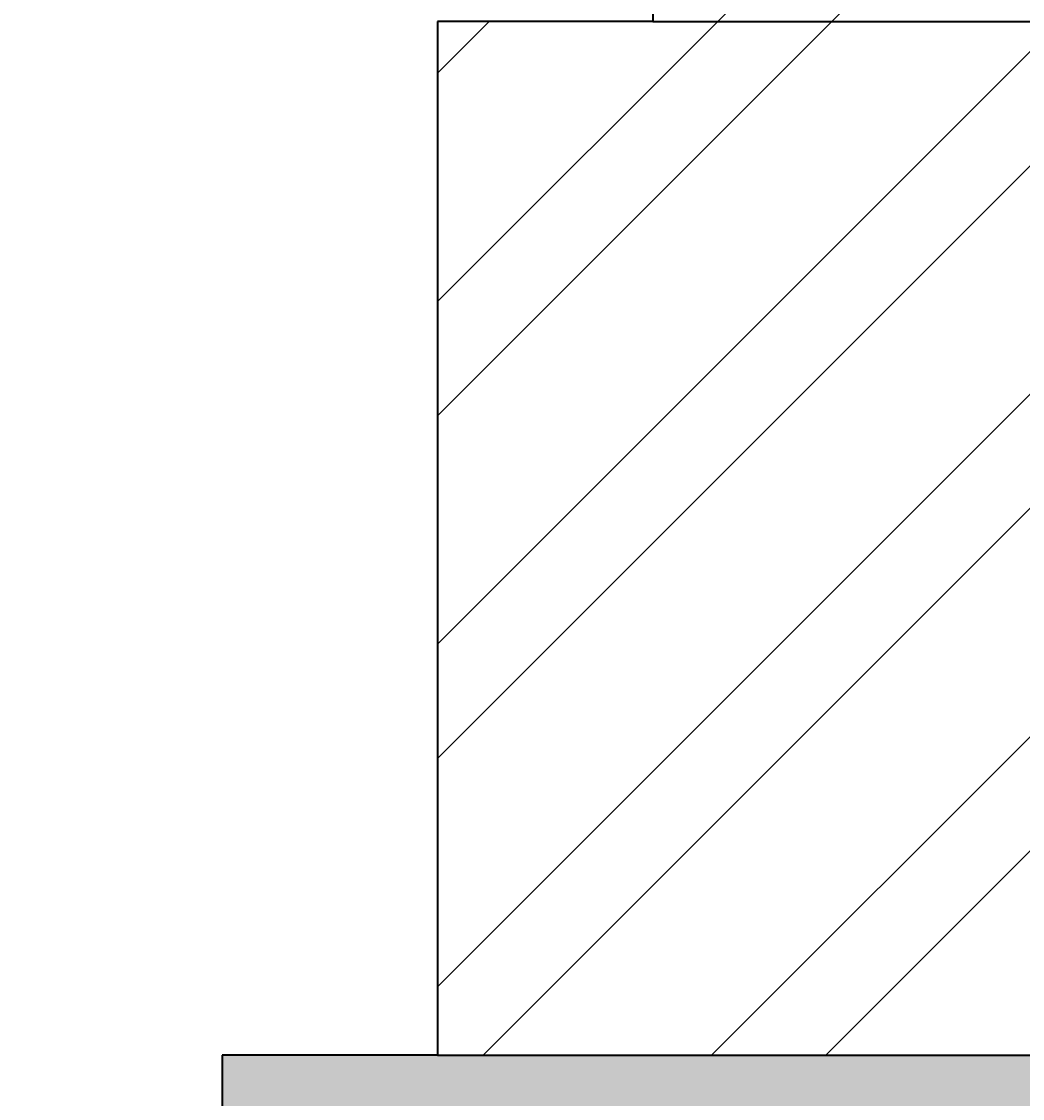
# Model space of a CAD drawing. Units: inches. Extents: x -301 to 715, y -607 to 364.
# Tile 5 of 141: x -66 to -43, y -536 to -511. Entities that reach past the tile are written whole.
import ezdxf

# ---------------------------------------------------------------- set-up
doc = ezdxf.new("R2010")
doc.units = ezdxf.units.IN
doc.header["$MEASUREMENT"] = 0
for name, color, linetype, lineweight in [('A-ANNO-DIMS', 2, 'Continuous', 18), ('A-SECT-PATT', 8, 'Continuous', 13), ('S-FNDN', 2, 'Continuous', 35)]:
    doc.layers.add(name, color=color, linetype=linetype, lineweight=lineweight)
doc.styles.get("Standard").update_dxf_attribs({"font": 'arial.ttf'})
doc.dimstyles.get("Standard").update_dxf_attribs({"dimtxt": 0.18, "dimasz": 0.18, "dimexe": 0.18, "dimexo": 0.0625, "dimgap": 0.09, "dimtad": 0, "dimtih": 1, "dimtoh": 1, "dimdec": 1, "dimzin": 0, "dimdsep": 46, "dimlunit": 4, "dimtxsty": 'Standard', "dimcen": 0.09, "dimclrd": 3, "dimclre": 4, "dimclrt": 6, "dimadec": 0, "dimazin": 0, "dimtfac": 1, "dimtdec": 1, "dimtofl": 0, "dimtmove": 0, "dimatfit": 3, "dimfxl": 1, "dimtfill": 2, "dimtfillclr": 51, "dimtolj": 1, "dimtzin": 0, "dimarcsym": 0})

# ---------------------------------------------------------------- blocks, each defined once
blk = doc.blocks.new('*D179')
at = {"layer": 'A-ANNO-DIMS', "color": 4, "lineweight": -2, "transparency": 16777216}
for p, q in [((-87.981, -433.54), (-87.981, -573.809)), ((-35.282, -463.54), (-35.282, -573.809))]:
    blk.add_line(p, q, dxfattribs=at)
at = {"layer": 'A-ANNO-DIMS', "color": 3, "lineweight": -2, "transparency": 16777216}
for p, q in [((-87.801, -573.629), (-62.174, -573.629)), ((-35.462, -573.629), (-61.089, -573.629))]:
    blk.add_line(p, q, dxfattribs=at)
at = {"layer": 'A-ANNO-DIMS', "color": 3, "transparency": 16777216}
for points in [[(-87.801, -573.599), (-87.801, -573.659), (-87.981, -573.629)], [(-35.462, -573.599), (-35.462, -573.659), (-35.282, -573.629)]]:
    blk.add_solid(points, dxfattribs=at)
at = {"layer": 'Defpoints', "color": 0, "transparency": 16777216}
for p in [(-87.981, -433.477), (-35.282, -463.477), (-35.282, -573.629)]:
    blk.add_point(p, dxfattribs=at)
at = {"layer": 'A-ANNO-DIMS', "color": 6, "transparency": 16777216, "insert": (-61.631, -573.629), "char_height": 0.18, "attachment_point": 5, "bg_fill": 1, "box_fill_scale": 1.25, "bg_fill_color": 51, "bg_fill_transparency": 0}
blk.add_mtext('\\A1;4\'-4 1/2"', dxfattribs=at)
blk = doc.blocks.new('*D191')
at = {"layer": 'A-ANNO-DIMS', "color": 4, "lineweight": -2, "transparency": 16777216}
for p, q in [((129.193, -481.477), (-266.112, -481.477)), ((114.193, -540.477), (-266.112, -540.477))]:
    blk.add_line(p, q, dxfattribs=at)
at = {"layer": 'A-ANNO-DIMS', "color": 3, "lineweight": -2, "transparency": 16777216}
for p, q in [((-265.932, -481.657), (-265.932, -510.797)), ((-265.932, -540.297), (-265.932, -511.158))]:
    blk.add_line(p, q, dxfattribs=at)
at = {"layer": 'A-ANNO-DIMS', "color": 3, "transparency": 16777216}
for points in [[(-265.962, -481.657), (-265.902, -481.657), (-265.932, -481.477)], [(-265.962, -540.297), (-265.902, -540.297), (-265.932, -540.477)]]:
    blk.add_solid(points, dxfattribs=at)
at = {"layer": 'Defpoints', "color": 0, "transparency": 16777216}
for p in [(129.255, -481.477), (-265.932, -540.477), (114.255, -540.477)]:
    blk.add_point(p, dxfattribs=at)
at = {"layer": 'A-ANNO-DIMS', "color": 6, "transparency": 16777216, "insert": (-265.932, -510.977), "char_height": 0.18, "attachment_point": 5, "bg_fill": 1, "box_fill_scale": 1.25, "bg_fill_color": 51, "bg_fill_transparency": 0}
blk.add_mtext('\\A1;4\'-11"', dxfattribs=at)

msp = doc.modelspace()

# ---------------------------------------------------------------- hatches: boundary and pattern name
at = {"layer": 'A-SECT-PATT'}
h = msp.add_hatch(dxfattribs=at)
h.set_pattern_fill('ANSI32', color=256, scale=15)
h.set_pattern_definition([(45, (10.321, 33.8764), (-3.977476, 3.977476), []), (45, (12.973, 33.8764), (-3.977476, 3.977476), [])])
h.paths.add_polyline_path([(-185.282, -324.477), (-199.282, -324.477), (-199.282, -329.477), (-194.282, -329.477), (-194.282, -353.477), (-185.282, -353.477)])
h.paths.add_polyline_path([(-185.282, -361.477), (-193.904, -361.477), (-193.982, -377.537), (-185.282, -377.537)])
h.paths.add_polyline_path([(143.218, -329.477), (148.218, -329.477), (148.218, -324.477), (134.255, -324.477), (134.255, -353.477), (143.218, -353.477)])
h.paths.add_polyline_path([(143.218, -361.477), (134.255, -361.477), (134.255, -377.477), (143.218, -377.477)])
h.paths.add_polyline_path([(-185.282, -439.477), (-194.282, -439.477), (-194.282, -463.477), (-185.282, -463.477)])
h.paths.add_polyline_path([(-185.282, -471.477), (-194.282, -471.477), (-194.282, -481.477), (-185.282, -481.477)])
h.paths.add_polyline_path([(-185.282, -463.477), (-194.282, -463.477), (-194.282, -466.477), (-185.282, -466.477)])
h.paths.add_polyline_path([(-185.282, -466.477), (-194.282, -466.477), (-194.282, -471.477), (-185.282, -471.477)])
h.paths.add_polyline_path([(-180.282, -481.477), (-185.282, -481.477), (-194.282, -481.477), (-199.282, -481.477), (-199.282, -493.477), (-180.282, -493.477)])
h.paths.add_polyline_path([(-175.282, -493.477), (-180.282, -493.477), (-199.282, -493.477), (-204.282, -493.477), (-204.282, -511.477), (-175.282, -511.477)])
h.paths.add_polyline_path([(-170.282, -511.477), (-175.282, -511.477), (-204.282, -511.477), (-209.282, -511.477), (-209.282, -535.477), (-170.282, -535.477)])
h.paths.add_polyline_path([(-35.282, -463.477), (-41.282, -463.477), (-41.282, -466.477), (-35.282, -466.477)])
h.paths.add_polyline_path([(-35.282, -466.477), (-41.282, -466.477), (-41.282, -471.477), (-35.282, -471.477)])
h.paths.add_polyline_path([(-35.282, -471.477), (-41.282, -471.477), (-41.282, -481.477), (-35.282, -481.477)])
h.paths.add_polyline_path([(-30.282, -481.477), (-46.282, -481.477), (-46.282, -493.477), (-30.282, -493.477)])
h.paths.add_polyline_path([(-25.282, -493.477), (-30.282, -493.477), (-46.282, -493.477), (-51.282, -493.477), (-51.282, -511.477), (-25.282, -511.477)])
h.paths.add_polyline_path([(-20.282, -511.477), (-25.282, -511.477), (-51.282, -511.477), (-56.282, -511.477), (-56.282, -535.477), (-20.282, -535.477)])
h.paths.add_polyline_path([(143.218, -463.477), (134.255, -463.477), (134.255, -466.477), (143.218, -466.477)])
h.paths.add_polyline_path([(143.218, -466.477), (134.255, -466.477), (134.255, -471.477), (143.218, -471.477)])
h.paths.add_polyline_path([(143.218, -471.477), (134.255, -471.477), (134.255, -481.477), (143.218, -481.477)])
h.paths.add_polyline_path([(148.255, -481.477), (143.255, -481.477), (134.255, -481.477), (129.255, -481.477), (129.255, -493.477), (148.255, -493.477)])
h.paths.add_polyline_path([(153.255, -493.477), (148.255, -493.477), (129.255, -493.477), (124.255, -493.477), (124.255, -511.477), (153.255, -511.477)])
h.paths.add_polyline_path([(158.255, -511.477), (153.255, -511.477), (124.255, -511.477), (119.255, -511.477), (119.255, -535.477), (158.255, -535.477)])
h = msp.add_hatch(dxfattribs=at)
h.set_pattern_fill('AR-CONC', color=256, scale=0.5)
h.set_pattern_definition([(50, (10.3213, 33.8764), (3.586301, -0.31376), [0.375, -4.125]), (355, (10.3213, 33.8764), (-0.693757, 3.76096), [0.3, -3.3]), (100.45144, (10.62, 33.8502), (2.892544, 3.4472), [0.3187, -3.50571]), (46.1842, (10.3213, 34.8764), (5.336207, -0.827596), [0.5625, -6.1875]), (96.6356, (10.766, 34.8074), (4.67331, 4.870593), [0.47805, -5.25857]), (351.1842, (10.321, 34.8764), (4.67331, 4.870593), [0.45, -4.95]), (21, (10.8213, 34.6264), (2.984535, -2.013094), [0.375, -4.125]), (326, (10.8213, 34.6264), (1.216577, 3.62575), [0.3, -3.3]), (71.45144, (11.07, 34.4586), (4.201112, 1.612656), [0.3187, -3.50571]), (37.5, (10.3213, 33.8764), (0.0607993, 1.6644693), [0, -3.26, 0, -3.35, 0, -3.3125]), (7.5, (10.3213, 33.8764), (1.3153477, 1.9720586), [0, -1.91, 0, -3.185, 0, -1.2625]), (327.5, (9.2063, 33.8764), (2.6691122, -0.1127744), [0, -1.25, 0, -3.9, 0, -5.175]), (317.5, (8.7063, 33.8764), (2.915931, 0.500525), [0, -1.625, 0, -2.59, 0, -3.675])])
h.paths.add_polyline_path([(-56.282, -535.477), (-61.282, -535.477), (-61.282, -540.477), (-15.282, -540.477), (-15.282, -535.477), (-20.282, -535.477)])
h.paths.add_polyline_path([(119.255, -535.477), (114.255, -535.477), (114.255, -540.477), (163.255, -540.477), (163.255, -535.477), (158.255, -535.477)])
h.paths.add_polyline_path([(-206.282, -471.477), (-209.282, -471.477), (-209.282, -481.477), (-206.282, -481.477), (-194.282, -481.477), (-194.282, -471.477)])
h.paths.add_polyline_path([(-41.282, -481.477), (-41.282, -471.477), (-185.282, -471.477), (-185.282, -481.477), (-180.282, -481.477)])
h.paths.add_polyline_path([(134.255, -481.477), (134.255, -471.477), (-35.282, -471.477), (-35.282, -481.477), (-30.282, -481.477)])
h.paths.add_polyline_path([(155.218, -481.477), (158.218, -481.477), (158.218, -471.477), (153.218, -471.477), (143.218, -471.477), (143.218, -481.477), (148.255, -481.477)])
h.paths.add_polyline_path([(-193.88, -356.477), (-193.904, -361.477), (143.218, -361.477), (143.218, -356.477)])

# ---------------------------------------------------------------- linework, layer by layer
at = {"layer": 'S-FNDN'}
for p, q in [((-51.282, -493.477), (-51.282, -511.477)), ((-51.282, -511.477), (-56.282, -511.477)), ((-56.282, -511.477), (-56.282, -535.477)), ((-51.282, -511.477), (-25.282, -511.477)), ((-56.282, -535.477), (-61.282, -535.477)), ((-61.282, -535.477), (-61.282, -540.477)), ((-56.282, -535.477), (-20.282, -535.477))]:
    msp.add_line(p, q, dxfattribs=at)

# ---------------------------------------------------------------- dimensions: what is measured, and where the dimension line sits
at = {"layer": 'A-ANNO-DIMS'}
dim = msp.add_linear_dim(base=(-35.282, -573.629), p1=(-87.981, -433.477), p2=(-35.282, -463.477), dimstyle='Standard', override={"dimdec": 1, "dimlfac": 1, "dimrnd": 0, "dimzin": 1, "dimdsep": 46, "dimlunit": 4, "dimfrac": 2}, dxfattribs=at)
dim.commit()
dim.dimension.update_dxf_attribs({"geometry": '*D179', "text_midpoint": (-61.631, -573.629)})
dim = msp.add_linear_dim(base=(-265.932, -540.477), p1=(129.255, -481.477), p2=(114.255, -540.477), angle=90, dimstyle='Standard', override={"dimdec": 1, "dimlfac": 1, "dimrnd": 0, "dimzin": 1, "dimdsep": 46, "dimlunit": 4, "dimfrac": 2}, dxfattribs=at)
dim.commit()
dim.dimension.update_dxf_attribs({"geometry": '*D191', "text_midpoint": (-265.932, -510.977)})

doc.saveas('drawing.dxf')
